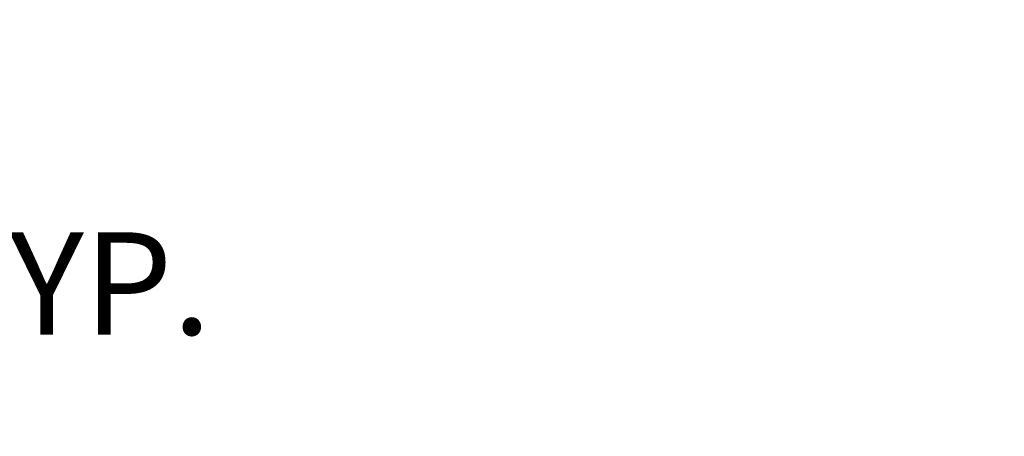
# Model space of a CAD drawing. Units: inches. Extents: x 73 to 1216, y -495 to 328.
# Tile 8 of 9: x 994 to 1167, y -28 to 45. Entities that reach past the tile are written whole.
import ezdxf

# ---------------------------------------------------------------- set-up
doc = ezdxf.new("R2010")
doc.units = ezdxf.units.IN
doc.layers.add('A-ANNO-DIMS', color=2, linetype='Continuous', lineweight=18)
doc.styles.get("Standard").update_dxf_attribs({"font": 'arial.ttf'})
doc.dimstyles.get("Standard").update_dxf_attribs({"dimtxt": 18, "dimasz": 12, "dimexe": 0.18, "dimexo": 0.0625, "dimgap": 0.09, "dimtad": 0, "dimtih": 1, "dimtoh": 1, "dimdec": 0, "dimzin": 0, "dimdsep": 46, "dimlunit": 3, "dimtxsty": 'Standard', "dimcen": 0.09, "dimadec": 0, "dimazin": 0, "dimtfac": 1, "dimtdec": 0, "dimtofl": 0, "dimtmove": 0, "dimatfit": 3, "dimfxl": 1, "dimtolj": 1, "dimtzin": 0, "dimarcsym": 0})

# ---------------------------------------------------------------- blocks, each defined once
blk = doc.blocks.new('*D38')
at = {"layer": 'A-ANNO-DIMS', "color": 0, "lineweight": -2, "transparency": 16777216}
for p, q in [((835.16, 83.11), (835.16, 69.65)), ((924.16, 83.11), (924.16, 69.65)), ((847.16, 69.83), (912.16, 69.83)), ((924.16, 69.83), (936.16, 69.83))]:
    blk.add_line(p, q, dxfattribs=at)
at = {"layer": 'A-ANNO-DIMS', "color": 0, "transparency": 16777216}
for points in [[(847.16, 71.83), (847.16, 67.83), (835.16, 69.83)], [(912.16, 71.83), (912.16, 67.83), (924.16, 69.83)]]:
    blk.add_solid(points, dxfattribs=at)
at = {"layer": 'Defpoints', "color": 0, "transparency": 16777216}
for p in [(835.16, 83.18), (924.16, 83.18), (924.16, 69.83)]:
    blk.add_point(p, dxfattribs=at)
at = {"layer": 'A-ANNO-DIMS', "color": 0, "transparency": 16777216, "insert": (1057.97, 69.83), "char_height": 18, "attachment_point": 5}
blk.add_mtext('\\A1;WARDROBE 89 TYP.', dxfattribs=at)
blk = doc.blocks.new('*D43')
at = {"layer": 'A-ANNO-DIMS', "color": 0, "lineweight": -2, "transparency": 16777216}
for p, q in [((903.36, 2.76), (903.36, -1.48)), ((919.39, 2.76), (919.39, -1.48)), ((891.36, -1.3), (879.36, -1.3)), ((931.39, -1.3), (943.39, -1.3))]:
    blk.add_line(p, q, dxfattribs=at)
at = {"layer": 'A-ANNO-DIMS', "color": 0, "transparency": 16777216}
for points in [[(891.36, 0.7), (891.36, -3.3), (903.36, -1.3)], [(931.39, 0.7), (931.39, -3.3), (919.39, -1.3)]]:
    blk.add_solid(points, dxfattribs=at)
at = {"layer": 'Defpoints', "color": 0, "transparency": 16777216}
for p in [(903.36, 2.82), (919.39, 2.82), (919.39, -1.3)]:
    blk.add_point(p, dxfattribs=at)
at = {"layer": 'A-ANNO-DIMS', "color": 0, "transparency": 16777216, "insert": (986.44, -1.3), "char_height": 18, "attachment_point": 5}
blk.add_mtext('\\A1;16 TYP.', dxfattribs=at)

msp = doc.modelspace()

# ---------------------------------------------------------------- dimensions: what is measured, and where the dimension line sits
at = {"layer": 'A-ANNO-DIMS'}
for base, p1, p2, text, picture, middle in [((924.1647, 69.8263), (835.1647, 83.1763), (924.1647, 83.1763), 'WARDROBE <> TYP.', '*D38', (1057.9696, 69.8263)), ((919.3873, -1.3024), (903.3556, 2.82), (919.3873, 2.82), '<> TYP.', '*D43', (986.4391, -1.3024))]:
    dim = msp.add_linear_dim(base=base, p1=p1, p2=p2, text=text, dimstyle='Standard', override={"dimdec": 0, "dimlfac": 1, "dimrnd": 0, "dimzin": 0, "dimdsep": 46, "dimlunit": 2}, dxfattribs=at)
    dim.commit()
    dim.dimension.update_dxf_attribs({"geometry": picture, "text_midpoint": middle})

doc.saveas('drawing.dxf')
